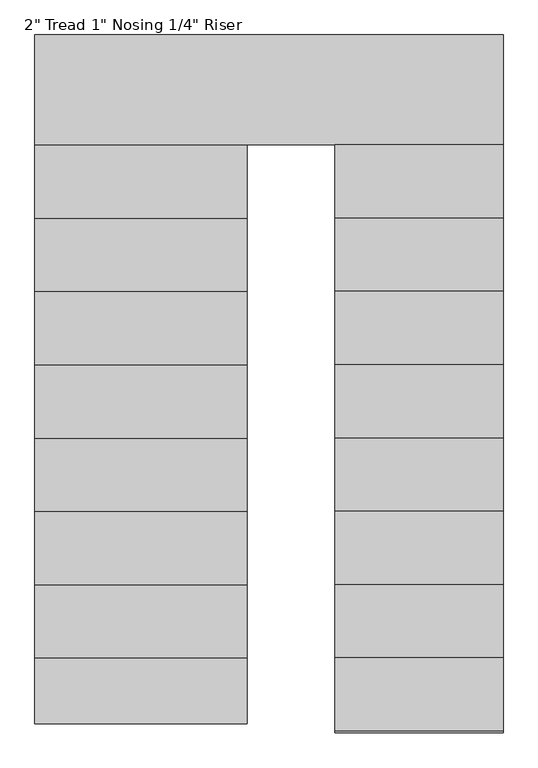
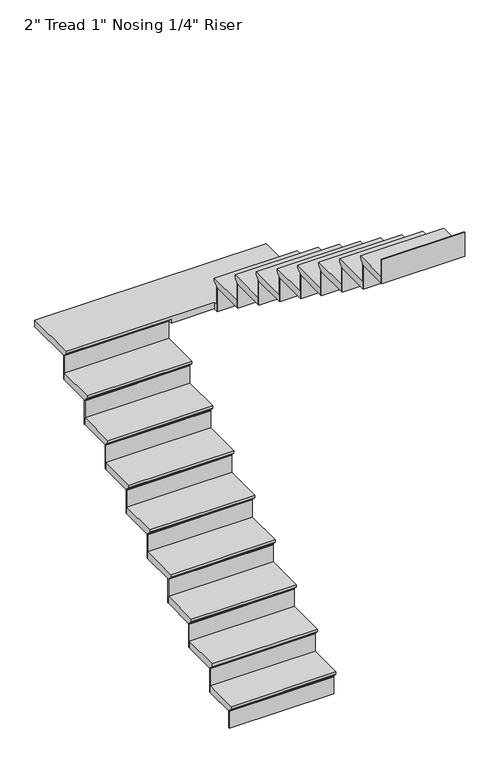
"""IFC4 building model written with IfcOpenShell, lengths in millimetres: stair flight geometry."""

from ifc_helpers import new_model, si_unit, origin, place, context, project, spatial, faceted_brep, source, transform, mapped, element, save


def stair_flight_00806837(model_context):
    return source(origin(), model_context, "Body", "Brep", [
        faceted_brep([(3394.0891134, -7650.9822004, 158.75), (3394.0891134, -7650.9822004, 177.8), (2657.4891134, -7650.9822004, 177.8), (2657.4891134, -7650.9822004, 158.75), (3394.0891134, -7625.5822004, 133.35), (2657.4891134, -7625.5822004, 133.35), (3394.0891134, -7396.9822004, 177.8), (2657.4891134, -7396.9822004, 177.8), (2657.4891134, -7625.5822004, 127.0), (2657.4891134, -7396.9822004, 127.0), (3394.0891134, -7396.9822004, 127.0), (3394.0891134, -7625.5822004, 127.0)], [[[0, 1, 2, 3]], [[4, 0, 3, 5]], [[2, 1, 6, 7]], [[8, 9, 10, 11]], [[2, 7, 9, 8, 5, 3]], [[8, 11, 4, 5]], [[6, 1, 0, 4, 11, 10]], [[7, 6, 10, 9]]]),
        faceted_brep([(3394.0891134, -7625.5822004, 127.0), (3394.0891134, -7625.5822004, 0.0), (3394.0891134, -7619.2322004, 0.0), (3394.0891134, -7619.2322004, 127.0), (2657.4891134, -7625.5822004, 127.0), (2657.4891134, -7619.2322004, 127.0), (2657.4891134, -7619.2322004, 0.0), (2657.4891134, -7625.5822004, 0.0)], [[[0, 1, 2, 3]], [[4, 5, 6, 7]], [[1, 0, 4, 7]], [[2, 1, 7, 6]], [[3, 2, 6, 5]], [[0, 3, 5, 4]]]),
        faceted_brep([(3394.0891134, -7396.9822004, 304.8), (3394.0891134, -7396.9822004, 127.0), (3394.0891134, -7390.6322004, 127.0), (3394.0891134, -7390.6322004, 304.8), (2657.4891134, -7396.9822004, 304.8), (2657.4891134, -7390.6322004, 304.8), (2657.4891134, -7390.6322004, 127.0), (2657.4891134, -7396.9822004, 127.0)], [[[0, 1, 2, 3]], [[4, 5, 6, 7]], [[1, 0, 4, 7]], [[2, 1, 7, 6]], [[3, 2, 6, 5]], [[0, 3, 5, 4]]]),
        faceted_brep([(2657.4891134, -7422.3822004, 355.6), (3394.0891134, -7422.3822004, 355.6), (3394.0891134, -7142.9822004, 355.6), (2657.4891134, -7142.9822004, 355.6), (2657.4891134, -7396.9822004, 304.8), (2657.4891134, -7142.9822004, 304.8), (3394.0891134, -7142.9822004, 304.8), (3394.0891134, -7396.9822004, 304.8), (2657.4891134, -7396.9822004, 311.15), (2657.4891134, -7422.3822004, 336.55), (3394.0891134, -7396.9822004, 311.15), (3394.0891134, -7422.3822004, 336.55)], [[[0, 1, 2, 3]], [[4, 5, 6, 7]], [[0, 3, 5, 4, 8, 9]], [[4, 7, 10, 8]], [[2, 1, 11, 10, 7, 6]], [[3, 2, 6, 5]], [[11, 1, 0, 9]], [[10, 11, 9, 8]]]),
        faceted_brep([(3394.0891134, -7142.9822004, 482.6), (3394.0891134, -7142.9822004, 304.8), (3394.0891134, -7136.6322004, 304.8), (3394.0891134, -7136.6322004, 482.6), (2657.4891134, -7142.9822004, 482.6), (2657.4891134, -7136.6322004, 482.6), (2657.4891134, -7136.6322004, 304.8), (2657.4891134, -7142.9822004, 304.8)], [[[0, 1, 2, 3]], [[4, 5, 6, 7]], [[1, 0, 4, 7]], [[2, 1, 7, 6]], [[3, 2, 6, 5]], [[0, 3, 5, 4]]]),
        faceted_brep([(2657.4891134, -7168.3822004, 533.4), (3394.0891134, -7168.3822004, 533.4), (3394.0891134, -6888.9822004, 533.4), (2657.4891134, -6888.9822004, 533.4), (2657.4891134, -7142.9822004, 482.6), (2657.4891134, -6888.9822004, 482.6), (3394.0891134, -6888.9822004, 482.6), (3394.0891134, -7142.9822004, 482.6), (2657.4891134, -7142.9822004, 488.95), (2657.4891134, -7168.3822004, 514.35), (3394.0891134, -7142.9822004, 488.95), (3394.0891134, -7168.3822004, 514.35)], [[[0, 1, 2, 3]], [[4, 5, 6, 7]], [[0, 3, 5, 4, 8, 9]], [[4, 7, 10, 8]], [[2, 1, 11, 10, 7, 6]], [[3, 2, 6, 5]], [[11, 1, 0, 9]], [[10, 11, 9, 8]]]),
        faceted_brep([(3394.0891134, -6888.9822004, 660.4), (3394.0891134, -6888.9822004, 482.6), (3394.0891134, -6882.6322004, 482.6), (3394.0891134, -6882.6322004, 660.4), (2657.4891134, -6888.9822004, 660.4), (2657.4891134, -6882.6322004, 660.4), (2657.4891134, -6882.6322004, 482.6), (2657.4891134, -6888.9822004, 482.6)], [[[0, 1, 2, 3]], [[4, 5, 6, 7]], [[1, 0, 4, 7]], [[2, 1, 7, 6]], [[3, 2, 6, 5]], [[0, 3, 5, 4]]]),
        faceted_brep([(2657.4891134, -6914.3822004, 711.2), (3394.0891134, -6914.3822004, 711.2), (3394.0891134, -6634.9822004, 711.2), (2657.4891134, -6634.9822004, 711.2), (2657.4891134, -6888.9822004, 660.4), (2657.4891134, -6634.9822004, 660.4), (3394.0891134, -6634.9822004, 660.4), (3394.0891134, -6888.9822004, 660.4), (2657.4891134, -6888.9822004, 666.75), (2657.4891134, -6914.3822004, 692.15), (3394.0891134, -6888.9822004, 666.75), (3394.0891134, -6914.3822004, 692.15)], [[[0, 1, 2, 3]], [[4, 5, 6, 7]], [[0, 3, 5, 4, 8, 9]], [[4, 7, 10, 8]], [[2, 1, 11, 10, 7, 6]], [[3, 2, 6, 5]], [[11, 1, 0, 9]], [[10, 11, 9, 8]]]),
        faceted_brep([(3394.0891134, -6634.9822004, 838.2), (3394.0891134, -6634.9822004, 660.4), (3394.0891134, -6628.6322004, 660.4), (3394.0891134, -6628.6322004, 838.2), (2657.4891134, -6634.9822004, 838.2), (2657.4891134, -6628.6322004, 838.2), (2657.4891134, -6628.6322004, 660.4), (2657.4891134, -6634.9822004, 660.4)], [[[0, 1, 2, 3]], [[4, 5, 6, 7]], [[1, 0, 4, 7]], [[2, 1, 7, 6]], [[3, 2, 6, 5]], [[0, 3, 5, 4]]]),
        faceted_brep([(2657.4891134, -6660.3822004, 889.0), (3394.0891134, -6660.3822004, 889.0), (3394.0891134, -6380.9822004, 889.0), (2657.4891134, -6380.9822004, 889.0), (2657.4891134, -6634.9822004, 838.2), (2657.4891134, -6380.9822004, 838.2), (3394.0891134, -6380.9822004, 838.2), (3394.0891134, -6634.9822004, 838.2), (2657.4891134, -6634.9822004, 844.55), (2657.4891134, -6660.3822004, 869.95), (3394.0891134, -6634.9822004, 844.55), (3394.0891134, -6660.3822004, 869.95)], [[[0, 1, 2, 3]], [[4, 5, 6, 7]], [[0, 3, 5, 4, 8, 9]], [[4, 7, 10, 8]], [[2, 1, 11, 10, 7, 6]], [[3, 2, 6, 5]], [[11, 1, 0, 9]], [[10, 11, 9, 8]]]),
        faceted_brep([(3394.0891134, -6380.9822004, 1016.0), (3394.0891134, -6380.9822004, 838.2), (3394.0891134, -6374.6322004, 838.2), (3394.0891134, -6374.6322004, 1016.0), (2657.4891134, -6380.9822004, 1016.0), (2657.4891134, -6374.6322004, 1016.0), (2657.4891134, -6374.6322004, 838.2), (2657.4891134, -6380.9822004, 838.2)], [[[0, 1, 2, 3]], [[4, 5, 6, 7]], [[1, 0, 4, 7]], [[2, 1, 7, 6]], [[3, 2, 6, 5]], [[0, 3, 5, 4]]]),
        faceted_brep([(2657.4891134, -6406.3822004, 1066.8), (3394.0891134, -6406.3822004, 1066.8), (3394.0891134, -6126.9822004, 1066.8), (2657.4891134, -6126.9822004, 1066.8), (2657.4891134, -6380.9822004, 1016.0), (2657.4891134, -6126.9822004, 1016.0), (3394.0891134, -6126.9822004, 1016.0), (3394.0891134, -6380.9822004, 1016.0), (2657.4891134, -6380.9822004, 1022.35), (2657.4891134, -6406.3822004, 1047.75), (3394.0891134, -6380.9822004, 1022.35), (3394.0891134, -6406.3822004, 1047.75)], [[[0, 1, 2, 3]], [[4, 5, 6, 7]], [[0, 3, 5, 4, 8, 9]], [[4, 7, 10, 8]], [[2, 1, 11, 10, 7, 6]], [[3, 2, 6, 5]], [[11, 1, 0, 9]], [[10, 11, 9, 8]]]),
        faceted_brep([(3394.0891134, -6126.9822004, 1193.8), (3394.0891134, -6126.9822004, 1016.0), (3394.0891134, -6120.6322004, 1016.0), (3394.0891134, -6120.6322004, 1193.8), (2657.4891134, -6126.9822004, 1193.8), (2657.4891134, -6120.6322004, 1193.8), (2657.4891134, -6120.6322004, 1016.0), (2657.4891134, -6126.9822004, 1016.0)], [[[0, 1, 2, 3]], [[4, 5, 6, 7]], [[1, 0, 4, 7]], [[2, 1, 7, 6]], [[3, 2, 6, 5]], [[0, 3, 5, 4]]]),
        faceted_brep([(2657.4891134, -6152.3822004, 1244.6), (3394.0891134, -6152.3822004, 1244.6), (3394.0891134, -5872.9822004, 1244.6), (2657.4891134, -5872.9822004, 1244.6), (2657.4891134, -6126.9822004, 1193.8), (2657.4891134, -5872.9822004, 1193.8), (3394.0891134, -5872.9822004, 1193.8), (3394.0891134, -6126.9822004, 1193.8), (2657.4891134, -6126.9822004, 1200.15), (2657.4891134, -6152.3822004, 1225.55), (3394.0891134, -6126.9822004, 1200.15), (3394.0891134, -6152.3822004, 1225.55)], [[[0, 1, 2, 3]], [[4, 5, 6, 7]], [[0, 3, 5, 4, 8, 9]], [[4, 7, 10, 8]], [[2, 1, 11, 10, 7, 6]], [[3, 2, 6, 5]], [[11, 1, 0, 9]], [[10, 11, 9, 8]]]),
        faceted_brep([(3394.0891134, -5872.9822004, 1371.6), (3394.0891134, -5872.9822004, 1193.8), (3394.0891134, -5866.6322004, 1193.8), (3394.0891134, -5866.6322004, 1371.6), (2657.4891134, -5872.9822004, 1371.6), (2657.4891134, -5866.6322004, 1371.6), (2657.4891134, -5866.6322004, 1193.8), (2657.4891134, -5872.9822004, 1193.8)], [[[0, 1, 2, 3]], [[4, 5, 6, 7]], [[1, 0, 4, 7]], [[2, 1, 7, 6]], [[3, 2, 6, 5]], [[0, 3, 5, 4]]]),
        faceted_brep([(2657.4891134, -5898.3822004, 1422.4), (3394.0891134, -5898.3822004, 1422.4), (3394.0891134, -5618.9822004, 1422.4), (2657.4891134, -5618.9822004, 1422.4), (2657.4891134, -5872.9822004, 1371.6), (2657.4891134, -5618.9822004, 1371.6), (3394.0891134, -5618.9822004, 1371.6), (3394.0891134, -5872.9822004, 1371.6), (2657.4891134, -5872.9822004, 1377.95), (2657.4891134, -5898.3822004, 1403.35), (3394.0891134, -5872.9822004, 1377.95), (3394.0891134, -5898.3822004, 1403.35)], [[[0, 1, 2, 3]], [[4, 5, 6, 7]], [[0, 3, 5, 4, 8, 9]], [[4, 7, 10, 8]], [[2, 1, 11, 10, 7, 6]], [[3, 2, 6, 5]], [[11, 1, 0, 9]], [[10, 11, 9, 8]]]),
        faceted_brep([(3394.0891134, -5618.9822004, 1549.4), (3394.0891134, -5618.9822004, 1371.6), (3394.0891134, -5612.6322004, 1371.6), (3394.0891134, -5612.6322004, 1549.4), (2657.4891134, -5618.9822004, 1549.4), (2657.4891134, -5612.6322004, 1549.4), (2657.4891134, -5612.6322004, 1371.6), (2657.4891134, -5618.9822004, 1371.6)], [[[0, 1, 2, 3]], [[4, 5, 6, 7]], [[1, 0, 4, 7]], [[2, 1, 7, 6]], [[3, 2, 6, 5]], [[0, 3, 5, 4]]]),
        faceted_brep([(4281.7311655, -5669.7822004, 1600.2), (4281.7311655, -5263.3822004, 1600.2), (2657.4891134, -5263.3822004, 1600.2), (2657.4891134, -5644.3822004, 1600.2), (3698.8891134, -5644.3822004, 1600.2), (3698.8891134, -5669.7822004, 1600.2), (4281.7311655, -5263.3822004, 1549.4), (4281.7311655, -5669.7822004, 1549.4), (3698.8891134, -5669.7822004, 1549.4), (3698.8891134, -5644.3822004, 1549.4), (3394.0891134, -5644.3822004, 1549.4), (3394.0891134, -5618.9822004, 1549.4), (2657.4891134, -5618.9822004, 1549.4), (2657.4891134, -5263.3822004, 1549.4), (3394.0891134, -5618.9822004, 1555.75), (2657.4891134, -5618.9822004, 1555.75), (2657.4891134, -5644.3822004, 1581.15), (3394.0891134, -5644.3822004, 1581.15)], [[[0, 1, 2, 3, 4, 5]], [[6, 7, 8, 9, 10, 11, 12, 13]], [[1, 0, 7, 6]], [[2, 1, 6, 13]], [[12, 11, 14, 15]], [[4, 3, 16, 17, 10, 9]], [[5, 4, 9, 8]], [[0, 5, 8, 7]], [[16, 15, 14, 17]], [[3, 2, 13, 12, 15, 16]], [[11, 10, 17, 14]]]),
        faceted_brep([(3698.8891134, -5669.7822004, 1727.2), (3698.8891134, -5669.7822004, 1549.4), (3698.8891134, -5676.1322004, 1549.4), (3698.8891134, -5676.1322004, 1727.2), (4281.7311655, -5669.7822004, 1727.2), (4281.7311655, -5676.1322004, 1727.2), (4281.7311655, -5676.1322004, 1549.4), (4281.7311655, -5669.7822004, 1549.4)], [[[0, 1, 2, 3]], [[4, 5, 6, 7]], [[1, 0, 4, 7]], [[2, 1, 7, 6]], [[3, 2, 6, 5]], [[0, 3, 5, 4]]]),
        faceted_brep([(4281.7311655, -5644.3822004, 1778.0), (3698.8891134, -5644.3822004, 1778.0), (3698.8891134, -5923.7822004, 1778.0), (4281.7311655, -5923.7822004, 1778.0), (4281.7311655, -5669.7822004, 1727.2), (4281.7311655, -5923.7822004, 1727.2), (3698.8891134, -5923.7822004, 1727.2), (3698.8891134, -5669.7822004, 1727.2), (4281.7311655, -5669.7822004, 1733.55), (4281.7311655, -5644.3822004, 1758.95), (3698.8891134, -5669.7822004, 1733.55), (3698.8891134, -5644.3822004, 1758.95)], [[[0, 1, 2, 3]], [[4, 5, 6, 7]], [[0, 3, 5, 4, 8, 9]], [[4, 7, 10, 8]], [[2, 1, 11, 10, 7, 6]], [[3, 2, 6, 5]], [[11, 1, 0, 9]], [[10, 11, 9, 8]]]),
        faceted_brep([(3698.8891134, -5923.7822004, 1905.0), (3698.8891134, -5923.7822004, 1727.2), (3698.8891134, -5930.1322004, 1727.2), (3698.8891134, -5930.1322004, 1905.0), (4281.7311655, -5923.7822004, 1905.0), (4281.7311655, -5930.1322004, 1905.0), (4281.7311655, -5930.1322004, 1727.2), (4281.7311655, -5923.7822004, 1727.2)], [[[0, 1, 2, 3]], [[4, 5, 6, 7]], [[1, 0, 4, 7]], [[2, 1, 7, 6]], [[3, 2, 6, 5]], [[0, 3, 5, 4]]]),
        faceted_brep([(4281.7311655, -5898.3822004, 1955.8), (3698.8891134, -5898.3822004, 1955.8), (3698.8891134, -6177.7822004, 1955.8), (4281.7311655, -6177.7822004, 1955.8), (4281.7311655, -5923.7822004, 1905.0), (4281.7311655, -6177.7822004, 1905.0), (3698.8891134, -6177.7822004, 1905.0), (3698.8891134, -5923.7822004, 1905.0), (4281.7311655, -5923.7822004, 1911.35), (4281.7311655, -5898.3822004, 1936.75), (3698.8891134, -5923.7822004, 1911.35), (3698.8891134, -5898.3822004, 1936.75)], [[[0, 1, 2, 3]], [[4, 5, 6, 7]], [[0, 3, 5, 4, 8, 9]], [[4, 7, 10, 8]], [[2, 1, 11, 10, 7, 6]], [[3, 2, 6, 5]], [[11, 1, 0, 9]], [[10, 11, 9, 8]]]),
        faceted_brep([(3698.8891134, -6177.7822004, 2082.8), (3698.8891134, -6177.7822004, 1905.0), (3698.8891134, -6184.1322004, 1905.0), (3698.8891134, -6184.1322004, 2082.8), (4281.7311655, -6177.7822004, 2082.8), (4281.7311655, -6184.1322004, 2082.8), (4281.7311655, -6184.1322004, 1905.0), (4281.7311655, -6177.7822004, 1905.0)], [[[0, 1, 2, 3]], [[4, 5, 6, 7]], [[1, 0, 4, 7]], [[2, 1, 7, 6]], [[3, 2, 6, 5]], [[0, 3, 5, 4]]]),
        faceted_brep([(4281.7311655, -6152.3822004, 2133.6), (3698.8891134, -6152.3822004, 2133.6), (3698.8891134, -6431.7822004, 2133.6), (4281.7311655, -6431.7822004, 2133.6), (4281.7311655, -6177.7822004, 2082.8), (4281.7311655, -6431.7822004, 2082.8), (3698.8891134, -6431.7822004, 2082.8), (3698.8891134, -6177.7822004, 2082.8), (4281.7311655, -6177.7822004, 2089.15), (4281.7311655, -6152.3822004, 2114.55), (3698.8891134, -6177.7822004, 2089.15), (3698.8891134, -6152.3822004, 2114.55)], [[[0, 1, 2, 3]], [[4, 5, 6, 7]], [[0, 3, 5, 4, 8, 9]], [[4, 7, 10, 8]], [[2, 1, 11, 10, 7, 6]], [[3, 2, 6, 5]], [[11, 1, 0, 9]], [[10, 11, 9, 8]]]),
        faceted_brep([(3698.8891134, -6431.7822004, 2260.6), (3698.8891134, -6431.7822004, 2082.8), (3698.8891134, -6438.1322004, 2082.8), (3698.8891134, -6438.1322004, 2260.6), (4281.7311655, -6431.7822004, 2260.6), (4281.7311655, -6438.1322004, 2260.6), (4281.7311655, -6438.1322004, 2082.8), (4281.7311655, -6431.7822004, 2082.8)], [[[0, 1, 2, 3]], [[4, 5, 6, 7]], [[1, 0, 4, 7]], [[2, 1, 7, 6]], [[3, 2, 6, 5]], [[0, 3, 5, 4]]]),
        faceted_brep([(4281.7311655, -6406.3822004, 2311.4), (3698.8891134, -6406.3822004, 2311.4), (3698.8891134, -6685.7822004, 2311.4), (4281.7311655, -6685.7822004, 2311.4), (4281.7311655, -6431.7822004, 2260.6), (4281.7311655, -6685.7822004, 2260.6), (3698.8891134, -6685.7822004, 2260.6), (3698.8891134, -6431.7822004, 2260.6), (4281.7311655, -6431.7822004, 2266.95), (4281.7311655, -6406.3822004, 2292.35), (3698.8891134, -6431.7822004, 2266.95), (3698.8891134, -6406.3822004, 2292.35)], [[[0, 1, 2, 3]], [[4, 5, 6, 7]], [[0, 3, 5, 4, 8, 9]], [[4, 7, 10, 8]], [[2, 1, 11, 10, 7, 6]], [[3, 2, 6, 5]], [[11, 1, 0, 9]], [[10, 11, 9, 8]]]),
        faceted_brep([(3698.8891134, -6685.7822004, 2438.4), (3698.8891134, -6685.7822004, 2260.6), (3698.8891134, -6692.1322004, 2260.6), (3698.8891134, -6692.1322004, 2438.4), (4281.7311655, -6685.7822004, 2438.4), (4281.7311655, -6692.1322004, 2438.4), (4281.7311655, -6692.1322004, 2260.6), (4281.7311655, -6685.7822004, 2260.6)], [[[0, 1, 2, 3]], [[4, 5, 6, 7]], [[1, 0, 4, 7]], [[2, 1, 7, 6]], [[3, 2, 6, 5]], [[0, 3, 5, 4]]]),
        faceted_brep([(4281.7311655, -6660.3822004, 2489.2), (3698.8891134, -6660.3822004, 2489.2), (3698.8891134, -6939.7822004, 2489.2), (4281.7311655, -6939.7822004, 2489.2), (4281.7311655, -6685.7822004, 2438.4), (4281.7311655, -6939.7822004, 2438.4), (3698.8891134, -6939.7822004, 2438.4), (3698.8891134, -6685.7822004, 2438.4), (4281.7311655, -6685.7822004, 2444.75), (4281.7311655, -6660.3822004, 2470.15), (3698.8891134, -6685.7822004, 2444.75), (3698.8891134, -6660.3822004, 2470.15)], [[[0, 1, 2, 3]], [[4, 5, 6, 7]], [[0, 3, 5, 4, 8, 9]], [[4, 7, 10, 8]], [[2, 1, 11, 10, 7, 6]], [[3, 2, 6, 5]], [[11, 1, 0, 9]], [[10, 11, 9, 8]]]),
        faceted_brep([(3698.8891134, -6939.7822004, 2616.2), (3698.8891134, -6939.7822004, 2438.4), (3698.8891134, -6946.1322004, 2438.4), (3698.8891134, -6946.1322004, 2616.2), (4281.7311655, -6939.7822004, 2616.2), (4281.7311655, -6946.1322004, 2616.2), (4281.7311655, -6946.1322004, 2438.4), (4281.7311655, -6939.7822004, 2438.4)], [[[0, 1, 2, 3]], [[4, 5, 6, 7]], [[1, 0, 4, 7]], [[2, 1, 7, 6]], [[3, 2, 6, 5]], [[0, 3, 5, 4]]]),
        faceted_brep([(4281.7311655, -6914.3822004, 2667.0), (3698.8891134, -6914.3822004, 2667.0), (3698.8891134, -7193.7822004, 2667.0), (4281.7311655, -7193.7822004, 2667.0), (4281.7311655, -6939.7822004, 2616.2), (4281.7311655, -7193.7822004, 2616.2), (3698.8891134, -7193.7822004, 2616.2), (3698.8891134, -6939.7822004, 2616.2), (4281.7311655, -6939.7822004, 2622.55), (4281.7311655, -6914.3822004, 2647.95), (3698.8891134, -6939.7822004, 2622.55), (3698.8891134, -6914.3822004, 2647.95)], [[[0, 1, 2, 3]], [[4, 5, 6, 7]], [[0, 3, 5, 4, 8, 9]], [[4, 7, 10, 8]], [[2, 1, 11, 10, 7, 6]], [[3, 2, 6, 5]], [[11, 1, 0, 9]], [[10, 11, 9, 8]]]),
        faceted_brep([(3698.8891134, -7193.7822004, 2794.0), (3698.8891134, -7193.7822004, 2616.2), (3698.8891134, -7200.1322004, 2616.2), (3698.8891134, -7200.1322004, 2794.0), (4281.7311655, -7193.7822004, 2794.0), (4281.7311655, -7200.1322004, 2794.0), (4281.7311655, -7200.1322004, 2616.2), (4281.7311655, -7193.7822004, 2616.2)], [[[0, 1, 2, 3]], [[4, 5, 6, 7]], [[1, 0, 4, 7]], [[2, 1, 7, 6]], [[3, 2, 6, 5]], [[0, 3, 5, 4]]]),
        faceted_brep([(4281.7311655, -7168.3822004, 2844.8), (3698.8891134, -7168.3822004, 2844.8), (3698.8891134, -7447.7822004, 2844.8), (4281.7311655, -7447.7822004, 2844.8), (4281.7311655, -7193.7822004, 2794.0), (4281.7311655, -7447.7822004, 2794.0), (3698.8891134, -7447.7822004, 2794.0), (3698.8891134, -7193.7822004, 2794.0), (4281.7311655, -7193.7822004, 2800.35), (4281.7311655, -7168.3822004, 2825.75), (3698.8891134, -7193.7822004, 2800.35), (3698.8891134, -7168.3822004, 2825.75)], [[[0, 1, 2, 3]], [[4, 5, 6, 7]], [[0, 3, 5, 4, 8, 9]], [[4, 7, 10, 8]], [[2, 1, 11, 10, 7, 6]], [[3, 2, 6, 5]], [[11, 1, 0, 9]], [[10, 11, 9, 8]]]),
        faceted_brep([(3698.8891134, -7447.7822004, 2971.8), (3698.8891134, -7447.7822004, 2794.0), (3698.8891134, -7454.1322004, 2794.0), (3698.8891134, -7454.1322004, 2971.8), (4281.7311655, -7447.7822004, 2971.8), (4281.7311655, -7454.1322004, 2971.8), (4281.7311655, -7454.1322004, 2794.0), (4281.7311655, -7447.7822004, 2794.0)], [[[0, 1, 2, 3]], [[4, 5, 6, 7]], [[1, 0, 4, 7]], [[2, 1, 7, 6]], [[3, 2, 6, 5]], [[0, 3, 5, 4]]]),
        faceted_brep([(3698.8891134, -7676.3822004, 3149.6), (3698.8891134, -7676.3822004, 2971.8), (3698.8891134, -7682.7322004, 2971.8), (3698.8891134, -7682.7322004, 3149.6), (4281.7311655, -7676.3822004, 3149.6), (4281.7311655, -7682.7322004, 3149.6), (4281.7311655, -7682.7322004, 2971.8), (4281.7311655, -7676.3822004, 2971.8)], [[[0, 1, 2, 3]], [[4, 5, 6, 7]], [[1, 0, 4, 7]], [[2, 1, 7, 6]], [[3, 2, 6, 5]], [[0, 3, 5, 4]]]),
        faceted_brep([(4281.7311655, -7422.3822004, 3022.6), (3698.8891134, -7422.3822004, 3022.6), (3698.8891134, -7676.3822004, 3022.6), (4281.7311655, -7676.3822004, 3022.6), (4281.7311655, -7447.7822004, 2971.8), (4281.7311655, -7676.3822004, 2971.8), (3698.8891134, -7676.3822004, 2971.8), (3698.8891134, -7447.7822004, 2971.8), (4281.7311655, -7447.7822004, 2978.15), (4281.7311655, -7422.3822004, 3003.55), (3698.8891134, -7447.7822004, 2978.15), (3698.8891134, -7422.3822004, 3003.55)], [[[0, 1, 2, 3]], [[4, 5, 6, 7]], [[0, 3, 5, 4, 8, 9]], [[4, 7, 10, 8]], [[2, 1, 11, 10, 7, 6]], [[3, 2, 6, 5]], [[11, 1, 0, 9]], [[10, 11, 9, 8]]]),
    ])


if __name__ == "__main__":
    model = new_model("IFC4")
    model_context = context("Model", 3, world=origin())
    ifc_project = project(units=[si_unit("LENGTHUNIT", "METRE", prefix="MILLI")], contexts=[model_context])
    site = spatial("IfcSite", under=ifc_project)
    building = spatial("IfcBuilding", under=site)
    placement = place(None, origin())
    stair_flight_shape = stair_flight_00806837(model_context)
    element("IfcStairFlight", 1, ObjectType="2\" Tread 1\" Nosing 1/4\" Riser", at=placement, inside=building, context=model_context, shape_type="MappedRepresentation", body=[
        mapped(stair_flight_shape, transform((0.0, 0.0, 0.0), x_axis=(1.0, 0.0, 0.0), y_axis=(0.0, 1.0, 0.0), z_axis=(0.0, 0.0, 1.0))),
    ])
    save(model, "model.ifc")
